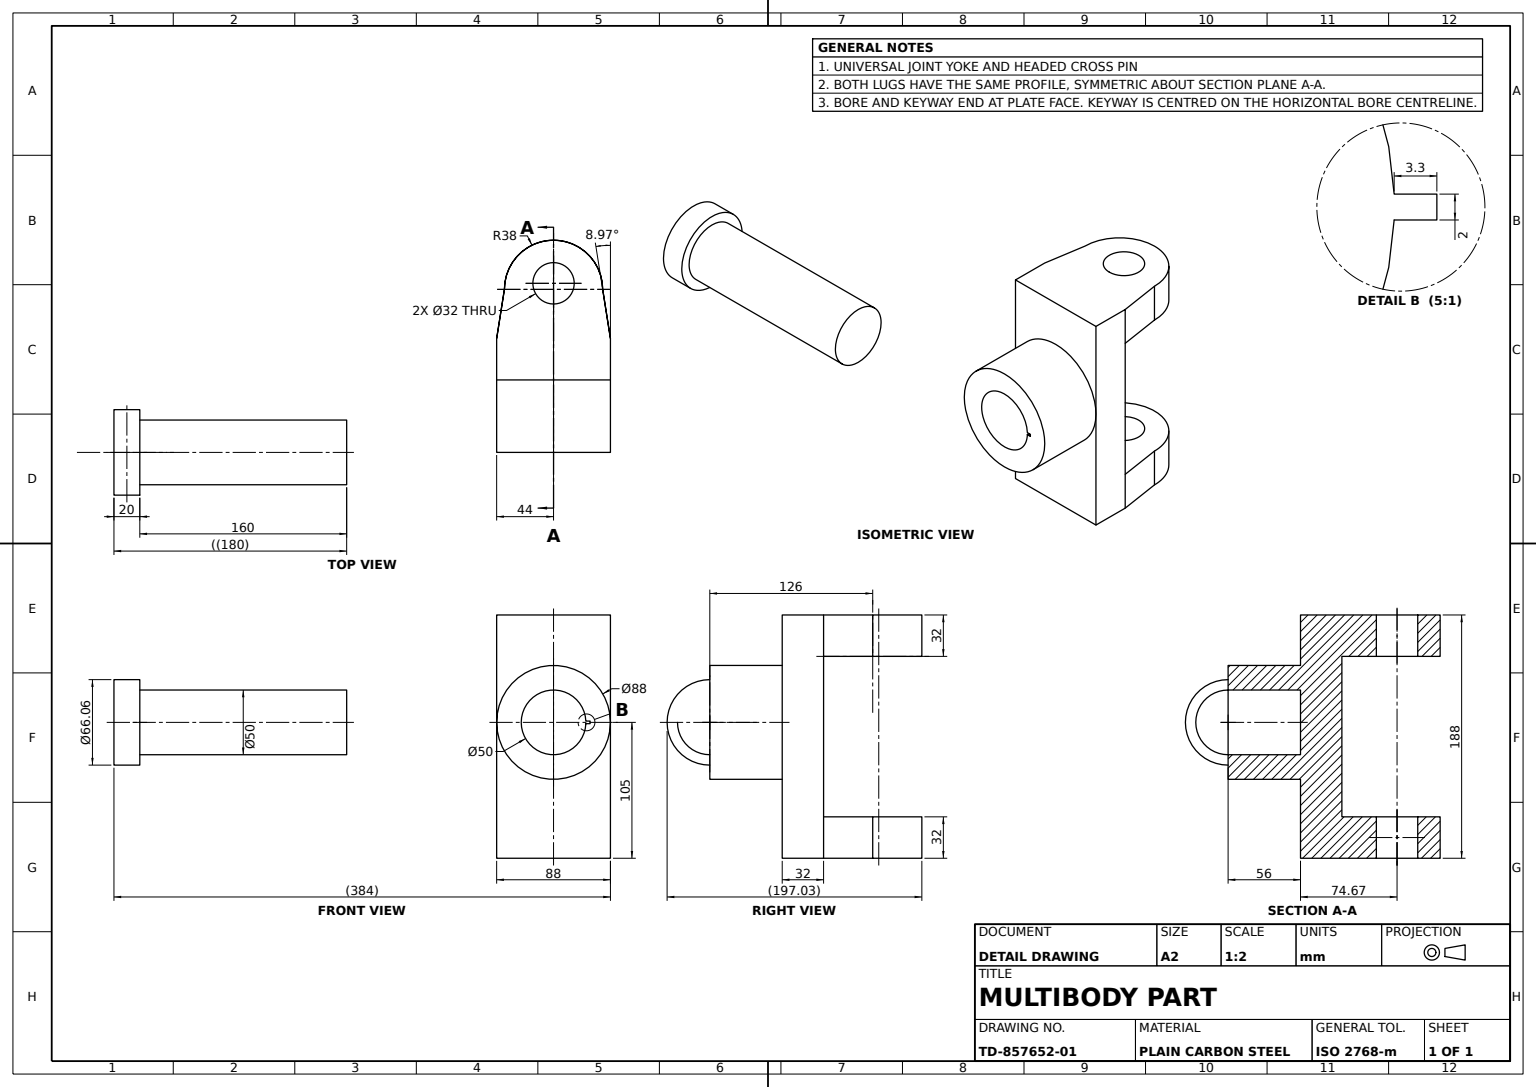
from build123d import *

# Parameters (mm, degrees)
HUB_PROFILE_88_R                  = 44
HUB_BOSS_88_DEPTH                 = 56
HUB_CUT_DEPTH                     = 56
YOKE_BASE_PLATE_DEPTH             = 32
YOKE_ARMS_DEPTH                   = 32
YOKE_START                        = -32
YOKE_WEB_DEPTH                    = 32
CROSS_PIN_BORE_PROFILE_R          = 16
CROSS_PIN_BORE_THROUGH_LUGS_DEPTH = 698
PIN_SHAFT_PROFILE_50_R            = 25
PIN_SHAFT_50_DEPTH                = 180
PIN_HEAD_PROFILE_R                = 33.029092334
PIN_HEAD_DEPTH                    = 20


with BuildPart() as part:
    # Hub Profile Ø88 → Hub Boss Ø88 (new body)
    with BuildSketch(Plane.XY):
        Circle(HUB_PROFILE_88_R)
    extrude(amount=HUB_BOSS_88_DEPTH)

    # Hub Cut Profile → Hub Cut (cut)
    with BuildSketch(Plane(origin=(0, 0, 0), x_dir=(-1, 0, 0), z_dir=(0, 0, -1))):
        with BuildLine():
            Line((24.98, -0.99979998), (28.282772946, -1.00020002))
            Line((28.282772946, -1.00020002), (28.282772946, 0.99979998))
            Line((28.282772946, 0.99979998), (24.98, 0.99979998))
            ThreePointArc((24.98, 0.99979998), (-25, 0), (24.98, -0.99979998))
        make_face()
    extrude(amount=-HUB_CUT_DEPTH, mode=Mode.SUBTRACT)

    # Yoke Base Profile → Yoke Base Plate (add)
    with BuildSketch(Plane.XY.offset(56)):
        Polygon((-44, 0), (-44, 83), (44, 83), (44, -105), (-44, -105), align=None)
    extrude(amount=YOKE_BASE_PLATE_DEPTH)

    # Yoke Arms Profile → Yoke Arms (add)
    with BuildSketch(Plane(origin=(0, 83, 0), x_dir=(1, 0, 0), z_dir=(0, 1, 0))):
        with BuildLine():
            Line((-44, -88), (44, -88))
            Line((44, -88), (38, -126))
            ThreePointArc((38, -126), (0, -164), (-38, -126))
            Line((-38, -126), (-44, -88))
        make_face()
    extrude(amount=-YOKE_ARMS_DEPTH)

    # Yoke Web Profile → Yoke Web (add)
    with BuildSketch(Plane.XZ.offset(105).offset(YOKE_START)):
        with BuildLine():
            Line((-38, 126), (-44, 88))
            Line((-44, 88), (44, 88))
            Line((44, 88), (38, 126))
            ThreePointArc((38, 126), (0, 164), (-38, 126))
        make_face()
    extrude(amount=YOKE_WEB_DEPTH)

    # Cross Pin Bore Profile → Cross Pin Bore Through Lugs (cut)
    with BuildSketch(Plane(origin=(0, 83, 0), x_dir=(1, 0, 0), z_dir=(0, 1, 0))):
        with Locations(Location((0, -130.667517764, 0), (0, 0, 270))):
            Circle(CROSS_PIN_BORE_PROFILE_R)
    extrude(amount=-CROSS_PIN_BORE_THROUGH_LUGS_DEPTH, mode=Mode.SUBTRACT)


with BuildPart() as body_2:
    # Pin Shaft Profile Ø50 → Pin Shaft Ø50 (new body)
    with BuildSketch(Plane(origin=(160, 0, 0), x_dir=(0, 0, -1), z_dir=(1, 0, 0))):
        with Locations(Location((0, 0, 0), (0, 0, 180))):
            Circle(PIN_SHAFT_PROFILE_50_R)
    extrude(amount=PIN_SHAFT_50_DEPTH)

    # Pin Head Profile → Pin Head (add)
    with BuildSketch(Plane(origin=(340, 0, 0), x_dir=(0, 0, -1), z_dir=(1, 0, 0))):
        Circle(PIN_HEAD_PROFILE_R)
    extrude(amount=-PIN_HEAD_DEPTH)


solid = Compound([part.part, body_2.part])
